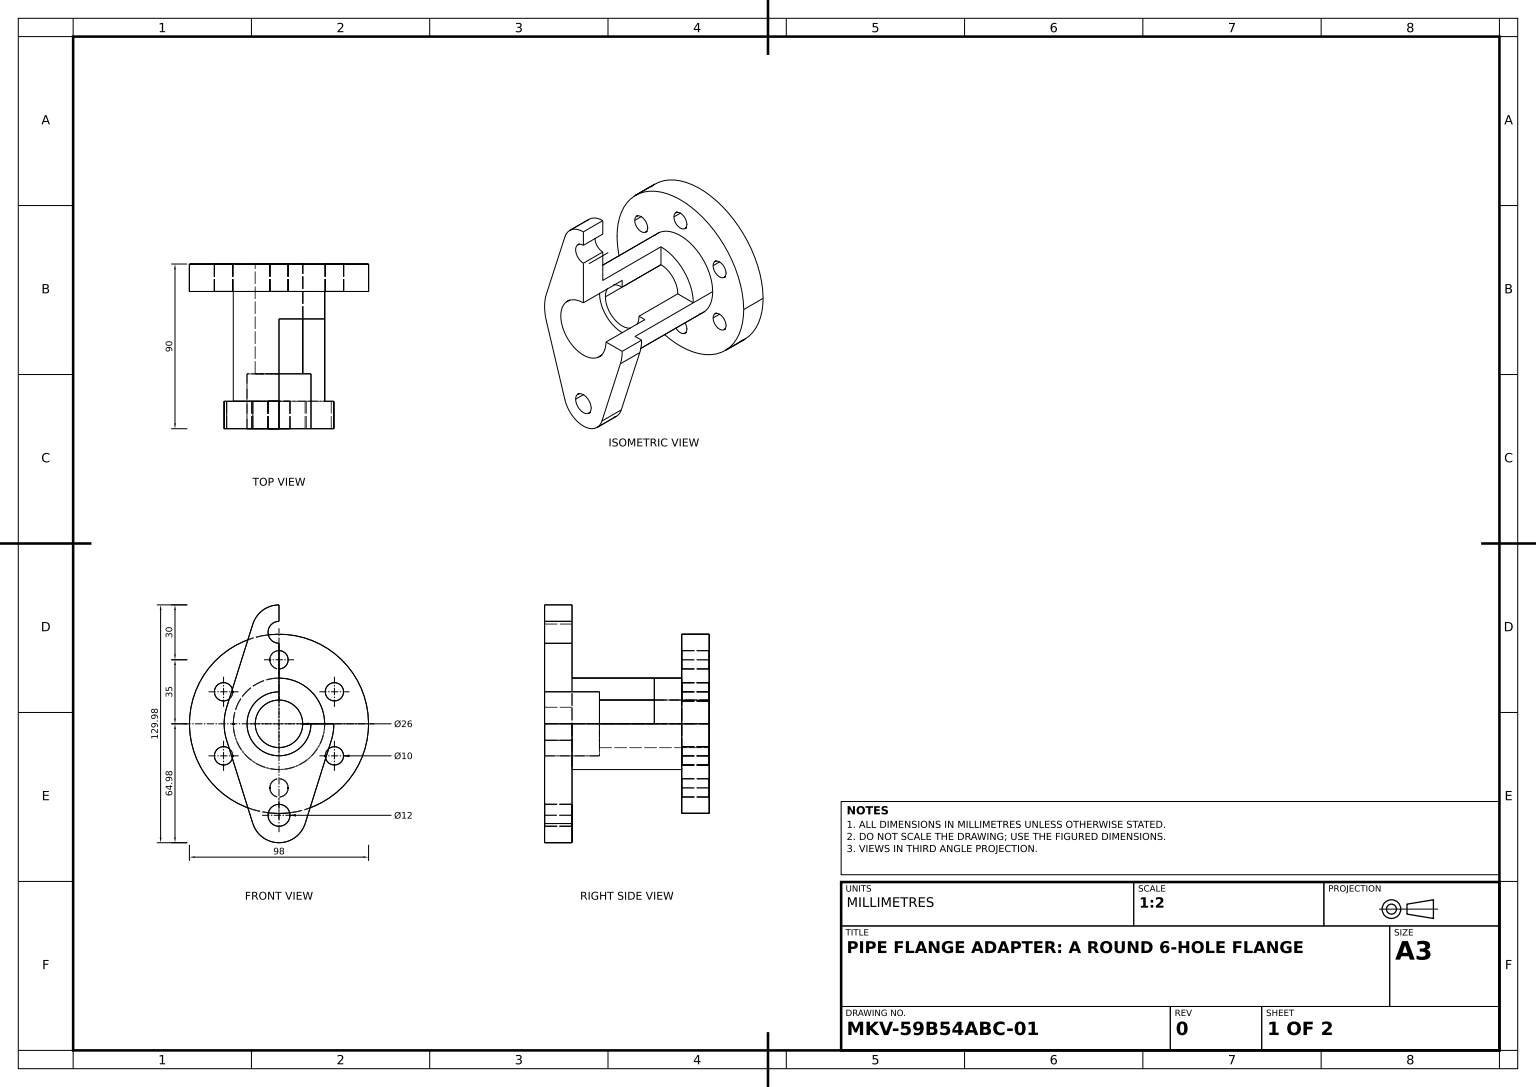
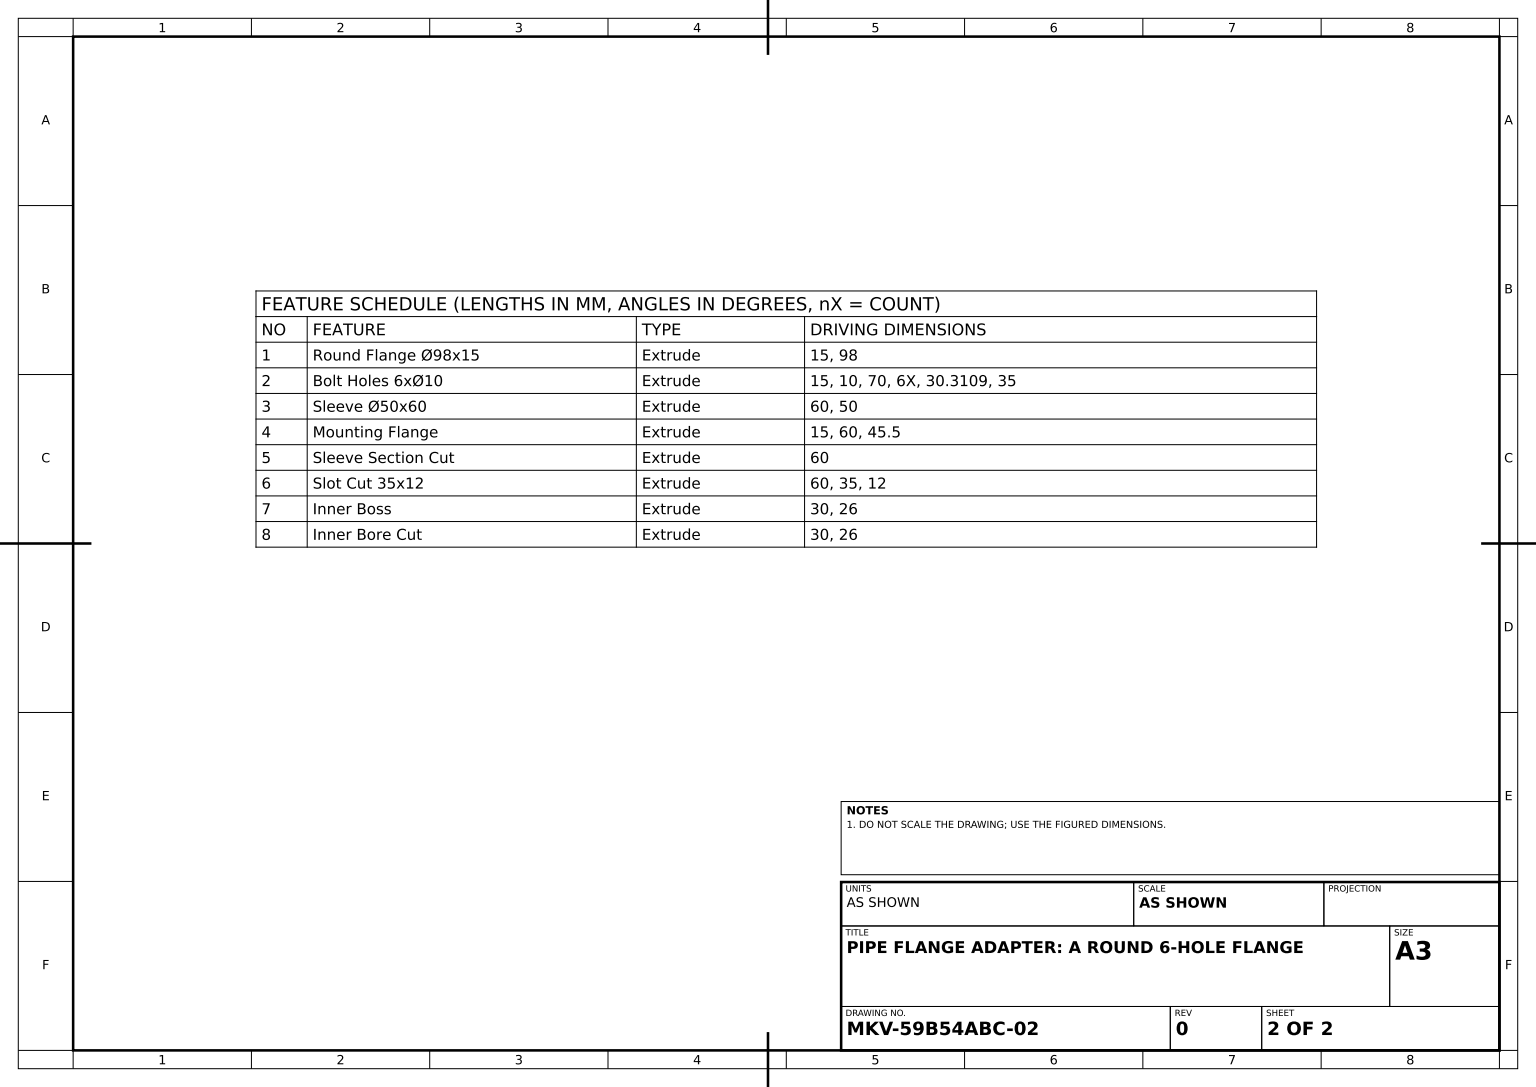
SolidWorks part; units mm, degrees
material "Plain Carbon Steel"
ref_plane "Front Plane" through (0, 0, 0) normal (0, 0, 1) x (1, 0, 0)
ref_plane "Top Plane" through (0, 0, 0) normal (0, 1, 0) x (1, 0, 0)
ref_plane "Right Plane" through (0, 0, 0) normal (1, 0, 0) x (0, 0, -1)
sketch "Round Flange Sketch Ø98" plane through (0, 0, 0) normal (0, 0, 1) x (1, 0, 0)
  circle A0 centre (0, 0) radius 49
  dimension "D1" = 98
extrude "Round Flange Ø98x15" add sketch "Round Flange Sketch Ø98" against normal blind 15
sketch "Bolt Holes Sketch 6xØ10 PCD70" plane through (0, 0, 0) normal (0, 0, 1) x (1, 0, 0)
  circle A0 centre (0, 0) radius 35 construction
  circle A1 centre (0, 35) radius 5
  circle A2 centre (30.3109, 17.5) radius 5
  circle A3 centre (30.3109, -17.5) radius 5
  circle A4 centre (0, -35) radius 5
  circle A5 centre (-30.3109, -17.5) radius 5
  circle A6 centre (-30.3109, 17.5) radius 5
  dimension "D1" = 10
  dimension "D2" = 70
  dimension "D4" = 30.3109
  dimension "D5" = 35
  dimension "D3" = 6
extrude "Bolt Holes 6xØ10" cut sketch "Bolt Holes Sketch 6xØ10 PCD70" against normal blind 15
sketch "Sleeve Sketch Ø50" plane through (0, 0, 0) normal (0, 0, 1) x (1, 0, 0)
  circle A0 centre (0, 0) radius 25
  dimension "D1" = 50
extrude "Sleeve Ø50x60" add sketch "Sleeve Sketch Ø50" along normal blind 60
sketch "Mounting Flange Sketch" plane through (0, 0, 60) normal (0, 0, 1) x (1, 0, 0)
  line L0 (0, 0) -> (0, -50) construction
  line L1 (0, 0) -> (49, 0) construction
  line L2 (-28.6182, -9) -> (-14.3091, -54.5)
  line L3 (28.6182, -9) -> (14.3091, -54.5)
  line L4 (-28.6182, 9) -> (-14.3091, 54.5)
  line L5 (28.6182, 9) -> (14.3091, 54.5)
  arc A1 (-28.6182, 9) -> (-28.6182, -9) centre (0, 0) ccw
  arc A3 (-14.3091, -54.5) -> (14.3091, -54.5) centre (0, -50) ccw
  circle A4 centre (0, 0) radius 49 construction
  arc A6 (-14.3091, 54.5) -> (14.3091, 54.5) centre (0, 50) cw
  arc A7 (28.6182, -9) -> (28.6182, 9) centre (0, 0) ccw
  dimension "D1" = 60
  dimension "D2" = 15
  dimension "D3" = 45.5
extrude "Mounting Flange" add sketch "Mounting Flange Sketch" along normal blind 15
sketch "Sleeve Section Cut Sketch" plane through (0, 0, 75) normal (0, 0, 1) x (1, 0, 0)
  line L0 (0, 65) -> (0, 0)
  line L1 (0, 0) -> (30, 0)
  line L2 (14.3091, 54.5) -> (28.6182, 9)
  arc A2 (14.3091, 54.5) -> (-14.3091, 54.5) centre (0, 50) ccw construction
  arc A3 (28.6182, -9) -> (28.6182, 9) centre (0, 0) ccw construction
  arc A4 (14.3091, 54.5) -> (0, 65) centre (0, 50) ccw
  arc A5 (28.6182, 9) -> (30, 0) centre (0, 0) cw
extrude "Sleeve Section Cut" cut sketch "Sleeve Section Cut Sketch" against normal blind 60
sketch "Slot Sketch 35x12" plane through (0, 0, 75) normal (0, 0, 1) x (1, 0, 0)
  line L0 (0, 0) -> (30, 0) construction
  circle A0 centre (0, 0) radius 17.5
  circle A2 centre (0, 50) radius 6
  circle A3 centre (0, -50) radius 6
  dimension "D1" = 35
  dimension "D2" = 12
extrude "Slot Cut 35x12" cut sketch "Slot Sketch 35x12" against normal blind 60
sketch "Inner Boss Sketch" plane through (0, 0, 15) normal (0, 0, 1) x (1, 0, 0)
  line L0 (0, 17.5) -> (0, 0)
  line L1 (0, 0) -> (17.5, 0)
  arc A0 (0, 13) -> (13, 0) centre (0, 0) ccw
  arc A1 (0, 17.5) -> (17.5, 0) centre (0, 0) ccw
  arc M2 (0, 17.5) -> (17.5, 0) centre (0, 0) ccw
  dimension "D2" = 26
extrude "Inner Boss" add sketch "Inner Boss Sketch" along normal blind 30 contours A0 L0 L1 M2
sketch "Inner Bore Sketch" plane through (0, 0, 15) normal (0, 0, 1) x (1, 0, 0)
  circle A0 centre (0, 0) radius 13
  dimension "D1" = 26
extrude "Inner Bore Cut" cut sketch "Inner Bore Sketch" against normal blind 30
